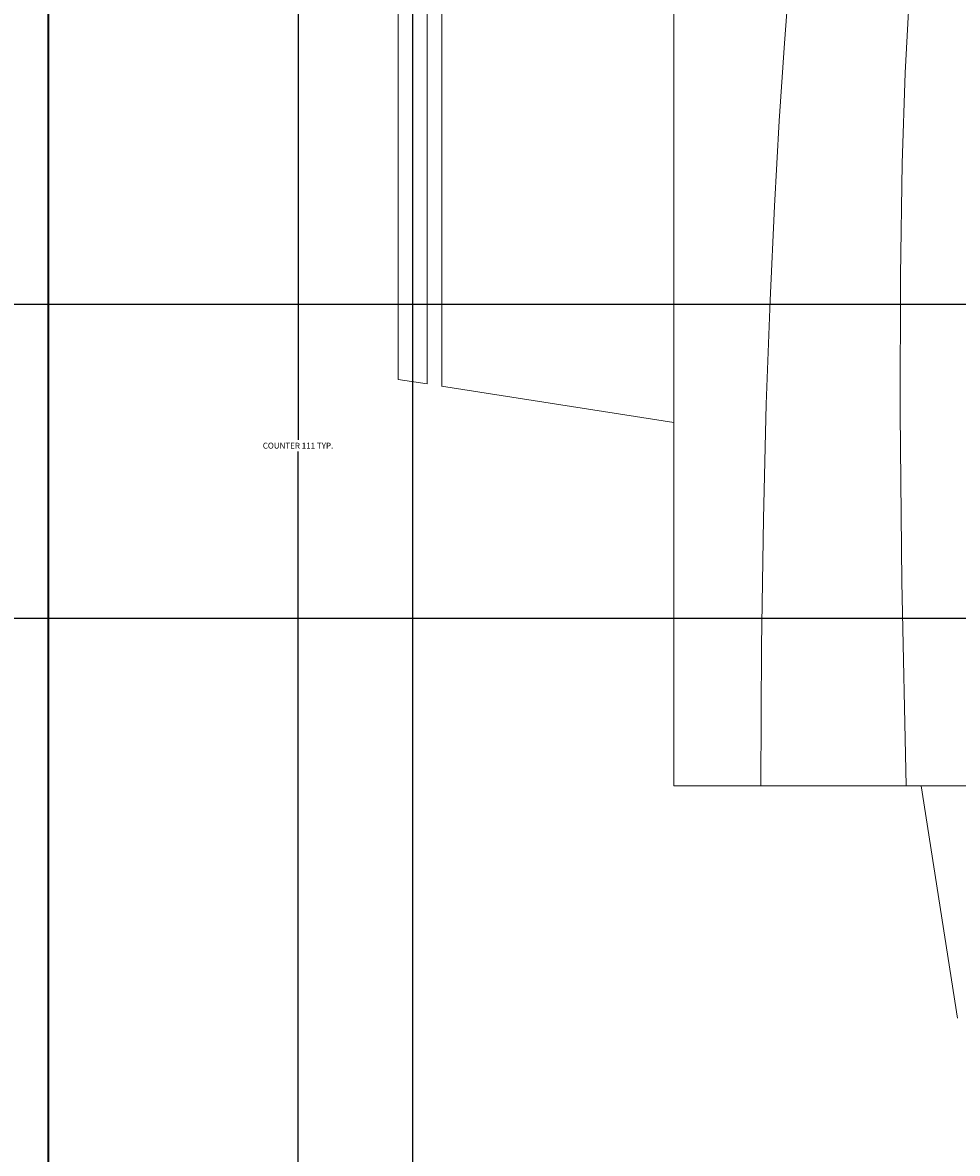
# Model space of a CAD drawing. Units: feet. Extents: x 1654 to 2985, y 1348 to 2230.
# Tile 25 of 53: x 1956 to 1985, y 1785 to 1820. Entities that reach past the tile are written whole.
import ezdxf

# ---------------------------------------------------------------- set-up
doc = ezdxf.new("R2010")
doc.units = ezdxf.units.FT
for name, color, linetype, lineweight in [('A-ANNO-DIMS', 2, 'Continuous', 18), ('A-FURN', 8, 'Continuous', 13), ('A-WALL', 7, 'Continuous', 35)]:
    doc.layers.add(name, color=color, linetype=linetype, lineweight=lineweight)
doc.styles.get("Standard").update_dxf_attribs({"font": 'arial.ttf'})
doc.dimstyles.get("Standard").update_dxf_attribs({"dimtxt": 0.18, "dimasz": 0.18, "dimexe": 0.18, "dimexo": 0.0625, "dimgap": 0.09, "dimtad": 0, "dimtih": 1, "dimtoh": 1, "dimdec": 4, "dimzin": 0, "dimdsep": 46, "dimtxsty": 'Standard', "dimcen": 0.09, "dimadec": 0, "dimazin": 0, "dimtfac": 1, "dimtdec": 4, "dimtofl": 0, "dimtmove": 0, "dimatfit": 3, "dimfxl": 1, "dimtolj": 1, "dimtzin": 0, "dimarcsym": 0})

# ---------------------------------------------------------------- blocks, each defined once
blk = doc.blocks.new('Dining Set - 36 x 72 in.')
for p, q in [((-22, 27.5), (-22.1562, 26.50042)), ((-22, 27.5), (-6, 27.5)), ((-5.8416, 26.5), (-22.1534, 26.5)), ((-22.2343, 26.00059), (-23.4847, 17.99762)), ((-22.2304, 26), (-5.7608, 26)), ((36, 18), (-36, 18)), ((-36, 18), (-36, -18)), ((-44.0006, 8.23428), (-35.9976, 9.48474))]:
    blk.add_line(p, q)
for points in [[(-36, 15), (-31.1772, 14.97754), (-26.8079, 14.91406), (-22.8538, 14.81543), (-19.276, 14.6875), (-16.0362, 14.53613), (-13.0957, 14.36718), (-10.4159, 14.18652), (-7.9583, 14)], [(-36, 10), (-28.9766, 10.14274), (-23.1725, 10.20442), (-18.4241, 10.19775), (-14.5677, 10.13541), (-11.4399, 10.03011), (-8.877, 9.89453)]]:
    blk.add_lwpolyline(points)
blk = doc.blocks.new('*D74')
at = {"layer": 'A-ANNO-DIMS', "color": 0, "lineweight": -2, "transparency": 16777216}
for p, q in [((1948.155, 1862.255), (1964.922, 1862.255)), ((1964.742, 1862.075), (1964.742, 1806.938)), ((1964.742, 1751.435), (1964.742, 1806.572)), ((1948.155, 1751.255), (1964.922, 1751.255))]:
    blk.add_line(p, q, dxfattribs=at)
at = {"layer": 'A-ANNO-DIMS', "color": 0, "transparency": 16777216}
for points in [[(1964.712, 1862.075), (1964.772, 1862.075), (1964.742, 1862.255)], [(1964.712, 1751.435), (1964.772, 1751.435), (1964.742, 1751.255)]]:
    blk.add_solid(points, dxfattribs=at)
at = {"layer": 'Defpoints', "color": 0, "transparency": 16777216}
for p in [(1948.092, 1862.255), (1964.742, 1862.255), (1948.092, 1751.255)]:
    blk.add_point(p, dxfattribs=at)
at = {"layer": 'A-ANNO-DIMS', "color": 0, "transparency": 16777216, "insert": (1964.742, 1806.755), "char_height": 0.18, "attachment_point": 5}
blk.add_mtext('\\A1;COUNTER 111 TYP.', dxfattribs=at)
blk = doc.blocks.new('*D91')
at = {"layer": 'A-ANNO-DIMS', "color": 0, "lineweight": -2, "transparency": 16777216}
for p, q in [((1852.155, 1801.468), (2242.272, 1801.468)), ((2242.092, 1801.288), (2242.092, 1776.544)), ((2242.092, 1751.435), (2242.092, 1776.18)), ((1852.155, 1751.255), (2242.272, 1751.255))]:
    blk.add_line(p, q, dxfattribs=at)
at = {"layer": 'A-ANNO-DIMS', "color": 0, "transparency": 16777216}
for points in [[(2242.062, 1801.288), (2242.122, 1801.288), (2242.092, 1801.468)], [(2242.062, 1751.435), (2242.122, 1751.435), (2242.092, 1751.255)]]:
    blk.add_solid(points, dxfattribs=at)
at = {"layer": 'Defpoints', "color": 0, "transparency": 16777216}
for p in [(1852.092, 1801.468), (2242.092, 1801.468), (1852.092, 1751.255)]:
    blk.add_point(p, dxfattribs=at)
at = {"layer": 'A-ANNO-DIMS', "color": 0, "transparency": 16777216, "insert": (2242.092, 1776.362), "char_height": 0.18, "attachment_point": 5}
blk.add_mtext('\\A1;50.21', dxfattribs=at)
blk = doc.blocks.new('*D97')
at = {"layer": 'A-ANNO-DIMS', "color": 0, "lineweight": -2, "transparency": 16777216}
for p, q in [((1957.092, 2108.192), (1957.092, 1534.075)), ((1968.254, 2108.192), (1968.254, 1534.075)), ((1957.272, 1534.255), (1962.219, 1534.255)), ((1968.074, 1534.255), (1963.128, 1534.255))]:
    blk.add_line(p, q, dxfattribs=at)
at = {"layer": 'A-ANNO-DIMS', "color": 0, "transparency": 16777216}
for points in [[(1957.272, 1534.285), (1957.272, 1534.225), (1957.092, 1534.255)], [(1968.074, 1534.285), (1968.074, 1534.225), (1968.254, 1534.255)]]:
    blk.add_solid(points, dxfattribs=at)
at = {"layer": 'Defpoints', "color": 0, "transparency": 16777216}
for p in [(1957.092, 2108.255), (1968.254, 2108.255), (1968.254, 1534.255)]:
    blk.add_point(p, dxfattribs=at)
at = {"layer": 'A-ANNO-DIMS', "color": 0, "transparency": 16777216, "insert": (1962.673, 1534.255), "char_height": 0.18, "attachment_point": 5}
blk.add_mtext('\\A1;11.162', dxfattribs=at)
blk = doc.blocks.new('*D98')
at = {"layer": 'A-ANNO-DIMS', "color": 0, "lineweight": -2, "transparency": 16777216}
for p, q in [((2061.03, 1811.081), (1811.912, 1811.081)), ((1812.092, 1810.901), (1812.092, 1781.35)), ((1812.092, 1751.435), (1812.092, 1780.986)), ((2061.03, 1751.255), (1811.912, 1751.255))]:
    blk.add_line(p, q, dxfattribs=at)
at = {"layer": 'A-ANNO-DIMS', "color": 0, "transparency": 16777216}
for points in [[(1812.062, 1810.901), (1812.122, 1810.901), (1812.092, 1811.081)], [(1812.062, 1751.435), (1812.122, 1751.435), (1812.092, 1751.255)]]:
    blk.add_solid(points, dxfattribs=at)
at = {"layer": 'Defpoints', "color": 0, "transparency": 16777216}
for p in [(1812.092, 1811.081), (2061.092, 1811.081), (2061.092, 1751.255)]:
    blk.add_point(p, dxfattribs=at)
at = {"layer": 'A-ANNO-DIMS', "color": 0, "transparency": 16777216, "insert": (1812.092, 1781.168), "char_height": 0.18, "attachment_point": 5}
blk.add_mtext('\\A1;59.83', dxfattribs=at)

msp = doc.modelspace()

# ---------------------------------------------------------------- linework, layer by layer
at = {"layer": 'A-WALL'}
msp.add_line((1957.0924, 1777.2549), (1957.0924, 1886.2549), dxfattribs=at)

# ---------------------------------------------------------------- block references
at = {"layer": 'A-FURN', "xscale": 0.8893748792417884, "yscale": 0.8893748792417884, "zscale": 0.8893748792417884, "rotation": 90}
msp.add_blockref('Dining Set - 36 x 72 in.', (1992.2681, 1828.3522), dxfattribs=at)

# ---------------------------------------------------------------- dimensions: what is measured, and where the dimension line sits
at = {"layer": 'A-ANNO-DIMS'}
dim = msp.add_linear_dim(base=(1968.2542, 1534.2549), p1=(1957.0924, 2108.2549), p2=(1968.2542, 2108.2549), dimstyle='Standard', override={"dimdec": 3, "dimlfac": 1, "dimrnd": 0, "dimzin": 0, "dimdsep": 46, "dimlunit": 2}, dxfattribs=at)
dim.commit()
dim.dimension.update_dxf_attribs({"geometry": '*D97', "text_midpoint": (1962.6733, 1534.2549)})
dim = msp.add_linear_dim(base=(1964.7424, 1862.2549), p1=(1948.0924, 1751.2549), p2=(1948.0924, 1862.2549), angle=90, text='COUNTER <> TYP.', dimstyle='Standard', override={"dimdec": 0, "dimlfac": 1, "dimrnd": 0, "dimzin": 0, "dimdsep": 46, "dimlunit": 2}, dxfattribs=at)
dim.commit()
dim.dimension.update_dxf_attribs({"geometry": '*D74', "text_midpoint": (1964.7424, 1806.7549)})
for base, p1, p2, picture, middle in [((1812.0924, 1811.0815), (2061.0924, 1751.2549), (2061.0924, 1811.0815), '*D98', (1812.0924, 1781.1682)), ((2242.0924, 1801.4683), (1852.0924, 1751.2549), (1852.0924, 1801.4683), '*D91', (2242.0924, 1776.3616))]:
    dim = msp.add_linear_dim(base=base, p1=p1, p2=p2, angle=90, dimstyle='Standard', override={"dimdec": 2, "dimlfac": 1, "dimrnd": 0, "dimzin": 0, "dimdsep": 46, "dimlunit": 2}, dxfattribs=at)
    dim.commit()
    dim.dimension.update_dxf_attribs({"geometry": picture, "text_midpoint": middle})

doc.saveas('drawing.dxf')
